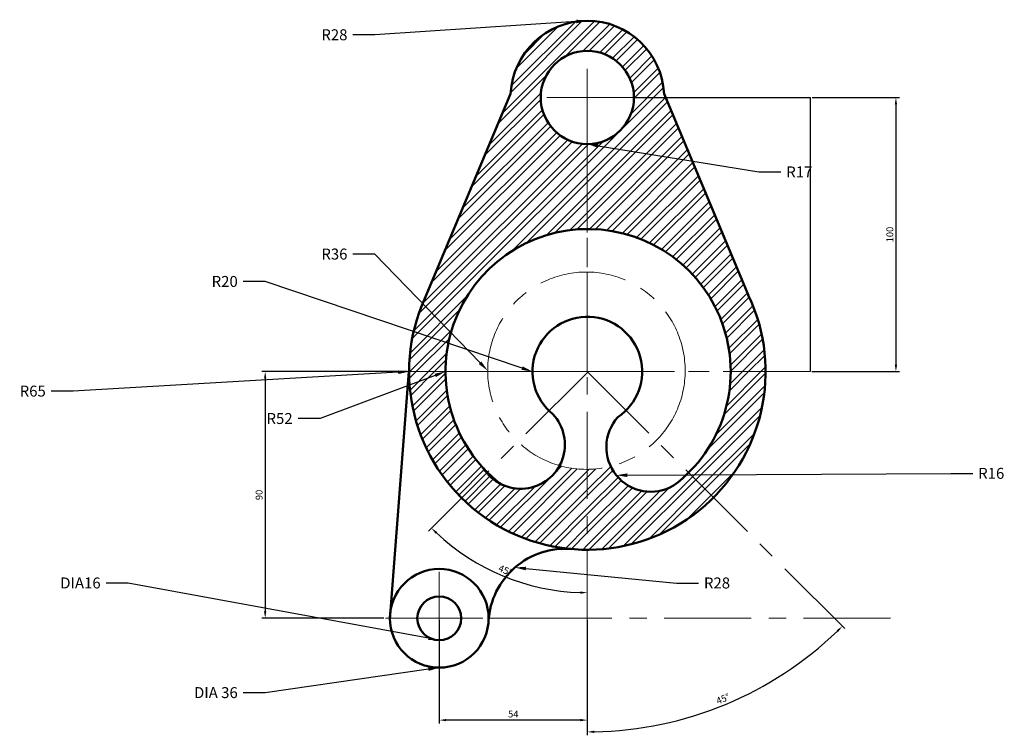
# Model space of a CAD drawing. Units: millimetres. Extents: x 3670 to 4030, y 1814 to 2076.
import ezdxf
from ezdxf import colors
from ezdxf.entities.mleader import LeaderData, LeaderLine
from ezdxf.math import Vec2, Vec3

# ---------------------------------------------------------------- set-up
doc = ezdxf.new("R2010")
doc.units = ezdxf.units.MM
doc.linetypes.add('CENTER', pattern=[50.8, 31.75, -6.35, 6.35, -6.35])
for name, color, linetype, lineweight in [('M-CNTR', 1, 'CENTER', 18), ('M-DIMS', 2, 'Continuous', 25), ('M-HATC', 8, 'Continuous', 18), ('M-OUTL', 7, 'Continuous', 50)]:
    doc.layers.add(name, color=color, linetype=linetype, lineweight=lineweight)
doc.styles.get("Standard").update_dxf_attribs({"font": 'arial.ttf'})
doc.dimstyles.new('ISO-25', dxfattribs={"dimtxt": 2.5, "dimasz": 2.5, "dimexe": 1.25, "dimexo": 0.625, "dimtad": 1, "dimtxsty": 'Standard', "dimcen": 2.5, "dimadec": 0, "dimazin": 0, "dimtfac": 1, "dimtmove": 0, "dimatfit": 3, "dimfxl": 1, "dimarcsym": 0})

# ---------------------------------------------------------------- blocks, each defined once
blk = doc.blocks.new('*D1')
at = {"layer": 'Defpoints', "color": 0, "transparency": 16777216}
for p in [(3877.47, 2034.06), (3877.47, 1947.15), (3949.01, 1875.7), (3877.47, 1854.64), (3911.52, 1820.19)]:
    blk.add_point(p, dxfattribs=at)
at = {"layer": 'M-DIMS', "color": 0, "lineweight": -2, "transparency": 16777216}
for p, q in [((3949.45, 1875.25), (3971.36, 1853.38)), ((3877.47, 1854.01), (3877.47, 1814.45))]:
    blk.add_line(p, q, dxfattribs=at)
blk.add_arc((3877.47, 1947.15), 131.45, 271.0897, 313.946, dxfattribs=at)
at = {"layer": 'M-DIMS', "color": 0, "transparency": 16777216}
for points in [[(3968.4, 1852.8), (3968.98, 1852.21), (3970.47, 1854.26)], [(3879.97, 1815.31), (3879.97, 1816.14), (3877.47, 1815.7)]]:
    blk.add_solid(points, dxfattribs=at)
at = {"layer": 'M-DIMS', "color": 0, "transparency": 16777216, "insert": (3927.08, 1827.48), "char_height": 2.5, "attachment_point": 5, "rotation": 22.5179}
blk.add_mtext('45°', dxfattribs=at)
blk = doc.blocks.new('*D2')
at = {"layer": 'Defpoints', "color": 0, "transparency": 16777216}
for p in [(3877.47, 2034.06), (3877.5, 1946.85), (3819.56, 1888.96), (3837.29, 1877.26), (3877.47, 1854.64)]:
    blk.add_point(p, dxfattribs=at)
at = {"layer": 'M-DIMS', "color": 0, "lineweight": -2, "transparency": 16777216}
blk.add_arc((3877.47, 1946.82), 80.33, 226.7608, 268.2168, dxfattribs=at)
at = {"layer": 'M-DIMS', "color": 0, "transparency": 16777216}
for points in [[(3822.15, 1888), (3822.73, 1888.6), (3820.64, 1890.04)], [(3874.98, 1866.95), (3874.96, 1866.11), (3877.47, 1866.49)]]:
    blk.add_solid(points, dxfattribs=at)
at = {"layer": 'M-DIMS', "color": 0, "transparency": 16777216, "insert": (3847.44, 1874.36), "char_height": 2.5, "attachment_point": 5, "rotation": 337.4888}
blk.add_mtext('45°', dxfattribs=at)
blk = doc.blocks.new('*D3')
at = {"layer": 'Defpoints', "color": 0, "transparency": 16777216}
for p in [(3958.78, 2047.15), (3958.75, 1947.15), (3990, 1947.15)]:
    blk.add_point(p, dxfattribs=at)
at = {"layer": 'M-DIMS', "color": 0, "lineweight": -2, "transparency": 16777216}
for p, q in [((3959.4, 2047.15), (3991.25, 2047.15)), ((3990, 2044.65), (3990, 1949.65)), ((3959.38, 1947.15), (3991.25, 1947.15))]:
    blk.add_line(p, q, dxfattribs=at)
at = {"layer": 'M-DIMS', "color": 0, "transparency": 16777216}
for points in [[(3989.58, 2044.65), (3990.42, 2044.65), (3990, 2047.15)], [(3989.58, 1949.65), (3990.42, 1949.65), (3990, 1947.15)]]:
    blk.add_solid(points, dxfattribs=at)
at = {"layer": 'M-DIMS', "color": 0, "transparency": 16777216, "insert": (3988.1, 1997.15), "char_height": 2.5, "attachment_point": 5, "rotation": 90}
blk.add_mtext('100', dxfattribs=at)
blk = doc.blocks.new('*D4')
at = {"layer": 'Defpoints', "color": 0, "transparency": 16777216}
for p in [(3812.44, 1947.14), (3760, 1857.15), (3803.9, 1857.15)]:
    blk.add_point(p, dxfattribs=at)
at = {"layer": 'M-DIMS', "color": 0, "lineweight": -2, "transparency": 16777216}
for p, q in [((3811.81, 1947.14), (3758.75, 1947.14)), ((3760, 1944.64), (3760, 1859.65)), ((3803.27, 1857.15), (3758.75, 1857.15))]:
    blk.add_line(p, q, dxfattribs=at)
at = {"layer": 'M-DIMS', "color": 0, "transparency": 16777216}
for points in [[(3759.58, 1944.64), (3760.42, 1944.64), (3760, 1947.14)], [(3759.58, 1859.65), (3760.42, 1859.65), (3760, 1857.15)]]:
    blk.add_solid(points, dxfattribs=at)
at = {"layer": 'M-DIMS', "color": 0, "transparency": 16777216, "insert": (3758.1, 1902.15), "char_height": 2.5, "attachment_point": 5, "rotation": 90}
blk.add_mtext('90', dxfattribs=at)
blk = doc.blocks.new('*D5')
at = {"layer": 'Defpoints', "color": 0, "transparency": 16777216}
for p in [(3823.47, 1857.15), (3877.47, 1857.15), (3823.47, 1820)]:
    blk.add_point(p, dxfattribs=at)
at = {"layer": 'M-DIMS', "color": 0, "lineweight": -2, "transparency": 16777216}
for p, q in [((3823.47, 1856.52), (3823.47, 1818.75)), ((3877.47, 1856.52), (3877.47, 1818.75)), ((3874.97, 1820), (3825.97, 1820))]:
    blk.add_line(p, q, dxfattribs=at)
at = {"layer": 'M-DIMS', "color": 0, "transparency": 16777216}
for points in [[(3825.97, 1820.42), (3825.97, 1819.58), (3823.47, 1820)], [(3874.97, 1820.42), (3874.97, 1819.58), (3877.47, 1820)]]:
    blk.add_solid(points, dxfattribs=at)
at = {"layer": 'M-DIMS', "color": 0, "transparency": 16777216, "insert": (3850.47, 1821.9), "char_height": 2.5, "attachment_point": 5}
blk.add_mtext('54', dxfattribs=at)

msp = doc.modelspace()

# ---------------------------------------------------------------- hatches: boundary and pattern name
at = {"layer": 'M-HATC'}
h = msp.add_hatch(dxfattribs=at)
h.set_pattern_fill('ANSI32', color=256, scale=0.5)
h.paths.add_polyline_path([(3877.469, 2030.149, -0.4142136), (3860.469, 2047.149, -1), (3894.469, 2047.149, -0.4142136), (3877.469, 2030.149), (3877.469, 1999.175, -0.4159692), (3929.753, 1947.149), (3942.469, 1947.149, 0.110279), (3936.296, 1974.796), (3905.435, 2048.538, 0.9522882), (3849.502, 2048.495), (3816.877, 1970.677, 0.0928618), (3812.469, 1947.149), (3825.753, 1947.149, -0.4127696), (3877.469, 1999.175)])
h = msp.add_hatch(dxfattribs=at)
h.set_pattern_fill('ANSI32', color=256, scale=0.5)
h.paths.add_polyline_path([(3825.753, 1947.149), (3812.469, 1947.149, 0.1997293), (3831.652, 1901.042), (3840.805, 1910.188, -0.0324169), (3839.573, 1911.874, -0.1886209)])
h = msp.add_hatch(dxfattribs=at)
h.set_pattern_fill('ANSI32', color=256, scale=0.5)
h.paths.add_polyline_path([(3942.469, 1947.149), (3929.753, 1947.149, -0.1997133), (3914.39, 1910.274), (3923.46, 1901.215, 0.1987504)])
h = msp.add_hatch(dxfattribs=at)
h.set_pattern_fill('ANSI32', color=256, scale=0.5)
h.paths.add_polyline_path([(3877.469, 1911.483, -0.071281), (3867.347, 1912.839, -0.5298711), (3840.805, 1910.188), (3831.652, 1901.042, 0.1980957), (3877.469, 1882.149)])
h = msp.add_hatch(dxfattribs=at)
h.set_pattern_fill('ANSI32', color=256, scale=0.5)
h.paths.add_polyline_path([(3923.46, 1901.215), (3914.39, 1910.274, -0.0346929), (3908.936, 1905.563, -0.4398285), (3885.981, 1912.583, -0.0598127), (3877.469, 1911.483), (3877.469, 1882.149, 0.1990744)])

# ---------------------------------------------------------------- linework, layer by layer
at = {"layer": 'M-CNTR'}
for p, q in [((3877.469, 2034.06), (3877.469, 2057.662)), ((3894.469, 2047.149), (3860.469, 2047.149)), ((3877.469, 1947.149), (3877.469, 2034.06)), ((3877.469, 2034.06), (3877.469, 1854.638)), ((3958.751, 1947.149), (3803.897, 1947.149)), ((3803.897, 1947.149), (3877.469, 1947.149)), ((3877.499, 1946.854), (3819.556, 1888.956)), ((3877.469, 1947.149), (3958.751, 1947.149)), ((3877.469, 1947.149), (3949.012, 1875.695)), ((3823.469, 1842.356), (3823.469, 1878.998)), ((3803.897, 1857.149), (3993.08, 1857.149)), ((3877.469, 1857.149), (3823.469, 1857.149)), ((3823.469, 1857.149), (3823.469, 1842.356))]:
    msp.add_line(p, q, dxfattribs=at)
msp.add_circle((3877.143, 1947.481), 36, dxfattribs=at)
at = {"layer": 'M-DIMS'}
for p, q in [((3894.526, 2047.146), (3958.775, 2047.146)), ((3958.68, 2047.146), (3958.68, 1947.146))]:
    msp.add_line(p, q, dxfattribs=at)
at = {"layer": 'M-OUTL'}
for p, q in [((3849.502, 2048.495), (3816.877, 1970.677)), ((3936.232, 1974.95), (3905.435, 2048.538)), ((3812.44, 1947.144), (3805.474, 1856.72))]:
    msp.add_line(p, q, dxfattribs=at)
for centre, radius in [((3877.469, 2047.149), 17), ((3823.469, 1857.149), 18), ((3823.469, 1857.149), 8)]:
    msp.add_circle(centre, radius, dxfattribs=at)
for centre, radius, start, end in [((3877.469, 2047.149), 28, 2.84354, 177.24367), ((3877.753, 1947.176), 52, 306.84531, 231.88878), ((3877.469, 1947.149), 65, 155.73056, 25.42107), ((3877.469, 1947.149), 20, 303.92024, 230.93176), ((3853.176, 1920.521), 16.119, 50.58681, 51.72913), ((3853.176, 1920.521), 16.119, 212.44224, 43.52121), ((3900.677, 1919.596), 16.283, 137.7141, 300.47733), ((3869.393, 1854.5), 28, 85.01804, 176.69912)]:
    msp.add_arc(centre, radius, start, end, dxfattribs=at)

# ---------------------------------------------------------------- dimensions: what is measured, and where the dimension line sits
at = {"layer": 'M-DIMS'}
for base, p1, p2, picture, middle in [((3990, 1947.149), (3958.775, 2047.146), (3958.751, 1947.149), '*D3', (3988.099, 1997.147)), ((3760, 1857.1486), (3812.4396, 1947.1444), (3803.8973, 1857.1486), '*D4', (3758.0986, 1902.1465))]:
    dim = msp.add_linear_dim(base=base, p1=p1, p2=p2, angle=90, dimstyle='ISO-25', override={"dimclrd": 0, "dimclre": 0, "dimclrt": 0}, dxfattribs=at)
    dim.commit()
    dim.dimension.update_dxf_attribs({"geometry": picture, "text_midpoint": middle})
for base, line1, line2, picture, middle in [((3837.285, 1877.265), ((3877.469, 2034.06), (3877.469, 1854.638)), ((3877.499, 1946.854), (3819.556, 1888.956)), '*D2', (3847.439, 1874.365)), ((3911.517, 1820.188), ((3877.469, 1947.149), (3949.012, 1875.695)), ((3877.469, 2034.06), (3877.469, 1854.638)), '*D1', (3927.083, 1827.475))]:
    dim = msp.add_angular_dim_2l(base=base, line1=line1, line2=line2, dimstyle='ISO-25', override={"dimclrd": 0, "dimclre": 0, "dimclrt": 0}, dxfattribs=at)
    dim.commit()
    dim.dimension.update_dxf_attribs({"geometry": picture, "text_midpoint": middle})
dim = msp.add_linear_dim(base=(3823.469, 1820), p1=(3877.469, 1857.149), p2=(3823.469, 1857.149), dimstyle='ISO-25', override={"dimclrd": 0, "dimclre": 0, "dimclrt": 0}, dxfattribs=at)
dim.commit()
dim.dimension.update_dxf_attribs({"geometry": '*D5', "text_midpoint": (3850.469, 1821.896)})

# ---------------------------------------------------------------- leaders
ml = msp.add_multileader_mtext('Standard', dxfattribs=at)
ml.set_content('R28', color=256)
ml.set_leader_properties()
ml.build(insert=Vec2(0, 0))
ctx = ml.context
ctx.base_point, ctx.plane_origin = Vec3(3778.434, 2070), Vec3(3877.448, 2075.149)
ctx.text_align_type = 2
notes = []
notes.append((ctx, [(0, (1, 1, 0), (3800, 2070), (-1, 0), 8, [(0, [(3877.448, 2075.149)], 0, [])])]))
ctx.mtext.insert, ctx.mtext.alignment, ctx.mtext.flow_direction = Vec3(3790, 2072.034), 3, 5
ml = msp.add_multileader_mtext('Standard', dxfattribs=at)
ml.set_content('R17', color=256)
ml.set_leader_properties()
ml.build(insert=Vec2(0, 0))
ctx = ml.context
ctx.base_point, ctx.plane_origin = Vec3(3948, 2020), Vec3(3877.469, 2030.149)
notes.append((ctx, [(0, (1, 1, 0), (3940, 2020), (1, 0), 8, [(0, [(3877.469, 2030.149)], 0, [])])]))
ctx.mtext.insert, ctx.mtext.flow_direction = Vec3(3950, 2022), 5
ml = msp.add_multileader_mtext('Standard', dxfattribs=at)
ml.set_content('R36', color=256)
ml.set_leader_properties()
ml.build(insert=Vec2(0, 0))
ctx = ml.context
ctx.base_point, ctx.plane_origin = Vec3(3778.445, 1990), Vec3(3841.143, 1947.481)
ctx.text_align_type = 2
notes.append((ctx, [(0, (1, 1, 0), (3800, 1990), (-1, 0), 8, [(0, [(3841.143, 1947.481)], 0, [])])]))
ctx.mtext.insert, ctx.mtext.alignment, ctx.mtext.flow_direction = Vec3(3790, 1992.035), 3, 5
ml = msp.add_multileader_mtext('Standard', dxfattribs=at)
ml.set_content('R20', color=256)
ml.set_leader_properties()
ml.build(insert=Vec2(0, 0))
ctx = ml.context
ctx.base_point, ctx.plane_origin = Vec3(3738.456, 1980), Vec3(3857.469, 1947.149)
ctx.text_align_type = 2
notes.append((ctx, [(0, (1, 1, 0), (3760, 1980), (-1, 0), 8, [(0, [(3857.469, 1947.149)], 0, [])])]))
ctx.mtext.insert, ctx.mtext.alignment, ctx.mtext.flow_direction = Vec3(3750, 1982.034), 3, 5
ml = msp.add_multileader_mtext('Standard', dxfattribs=at)
ml.set_content('R65', color=256)
ml.set_leader_properties()
ml.build(insert=Vec2(0, 0))
ctx = ml.context
ctx.base_point, ctx.plane_origin = Vec3(3668.412, 1940), Vec3(3812.469, 1947.149)
ctx.text_align_type = 2
notes.append((ctx, [(0, (1, 1, 0), (3690, 1940), (-1, 0), 8, [(0, [(3812.469, 1947.149)], 0, [])])]))
ctx.mtext.insert, ctx.mtext.alignment, ctx.mtext.flow_direction = Vec3(3680, 1942.034), 3, 5
ml = msp.add_multileader_mtext('Standard', dxfattribs=at)
ml.set_content('R52', color=256)
ml.set_leader_properties()
ml.build(insert=Vec2(0, 0))
ctx = ml.context
ctx.base_point, ctx.plane_origin = Vec3(3758.483, 1930), Vec3(3825.753, 1947.176)
ctx.text_align_type = 2
notes.append((ctx, [(0, (1, 1, 0), (3780, 1930), (-1, 0), 8, [(0, [(3825.753, 1947.176)], 0, [])])]))
ctx.mtext.insert, ctx.mtext.alignment, ctx.mtext.flow_direction = Vec3(3770, 1932.034), 3, 5
ml = msp.add_multileader_mtext('Standard', dxfattribs=at)
ml.set_content('R16', color=256)
ml.set_leader_properties()
ml.build(insert=Vec2(0, 0))
ctx = ml.context
ctx.base_point, ctx.plane_origin = Vec3(4018, 1910), Vec3(3888.039, 1909.328)
notes.append((ctx, [(0, (1, 1, 0), (4010, 1910), (1, 0), 8, [(0, [(3888.039, 1909.328)], 0, [])])]))
ctx.mtext.insert, ctx.mtext.flow_direction = Vec3(4020, 1912.034), 5
ml = msp.add_multileader_mtext('Standard', dxfattribs=at)
ml.set_content('R28', color=256)
ml.set_leader_properties()
ml.build(insert=Vec2(0, 0))
ctx = ml.context
ctx.base_point, ctx.plane_origin = Vec3(3918, 1870), Vec3(3851.076, 1875.677)
notes.append((ctx, [(0, (1, 1, 0), (3910, 1870), (1, 0), 8, [(0, [(3851.076, 1875.677)], 0, [])])]))
ctx.mtext.insert, ctx.mtext.flow_direction = Vec3(3920, 1872.034), 5
ml = msp.add_multileader_mtext('Standard', dxfattribs=at)
ml.set_content('DIA16', color=256)
ml.set_leader_properties()
ml.build(insert=Vec2(0, 0))
ctx = ml.context
ctx.base_point, ctx.plane_origin = Vec3(3683.157, 1870), Vec3(3823.469, 1849.149)
ctx.text_align_type = 2
notes.append((ctx, [(0, (1, 1, 0), (3710, 1870), (-1, 0), 8, [(0, [(3823.469, 1849.149)], 0, [])])]))
ctx.mtext.insert, ctx.mtext.alignment, ctx.mtext.flow_direction = Vec3(3700, 1872.034), 3, 5
ml = msp.add_multileader_mtext('Standard', dxfattribs=at)
ml.set_content('DIA 36', color=256)
ml.set_leader_properties()
ml.build(insert=Vec2(0, 0))
ctx = ml.context
ctx.base_point, ctx.plane_origin = Vec3(3731.604, 1830), Vec3(3823.469, 1839.149)
ctx.text_align_type = 2
notes.append((ctx, [(0, (1, 1, 0), (3760, 1830), (-1, 0), 8, [(0, [(3823.469, 1839.149)], 0, [])])]))
ctx.mtext.insert, ctx.mtext.alignment, ctx.mtext.flow_direction = Vec3(3750, 1832.035), 3, 5
for ctx, leaders in notes:
    for number, flags, end, landing, length, lines in leaders:
        leader = LeaderData()
        leader.index, (leader.has_last_leader_line, leader.has_dogleg_vector, leader.attachment_direction) = number, flags
        leader.last_leader_point, leader.dogleg_vector, leader.dogleg_length = Vec3(end), Vec3(landing), length
        for number, points, colour, breaks in lines:
            line = LeaderLine()
            line.index, line.vertices, line.color, line.breaks = number, Vec3.list(points), colors.encode_raw_color(colour), breaks
            leader.lines.append(line)
        ctx.leaders.append(leader)

doc.saveas('drawing.dxf')
